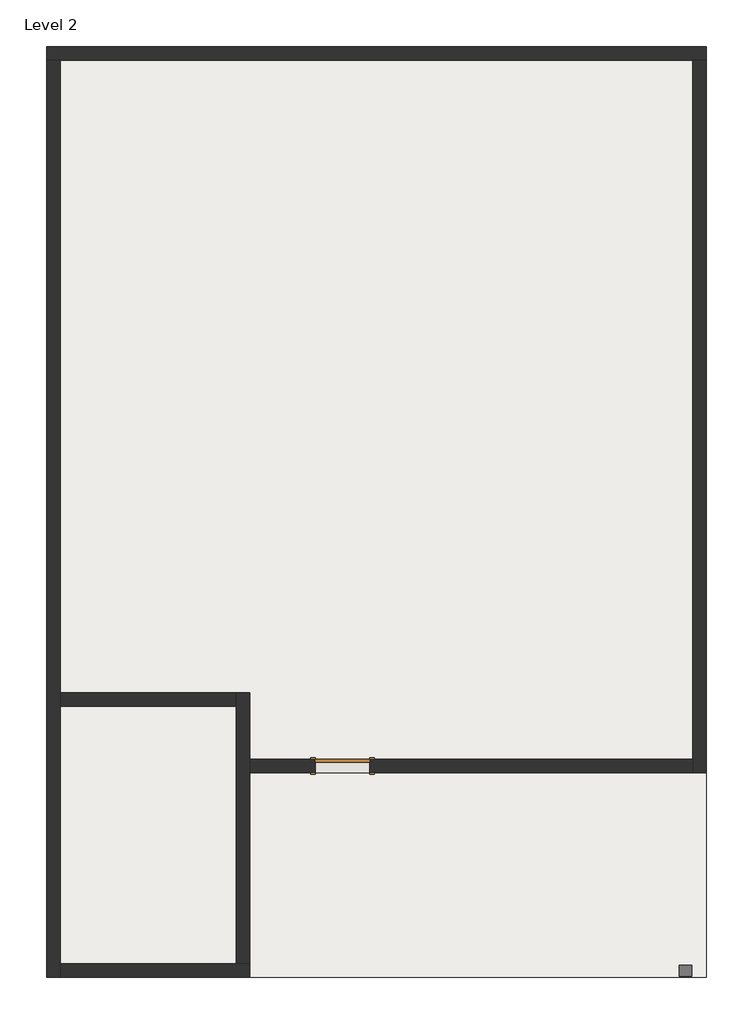
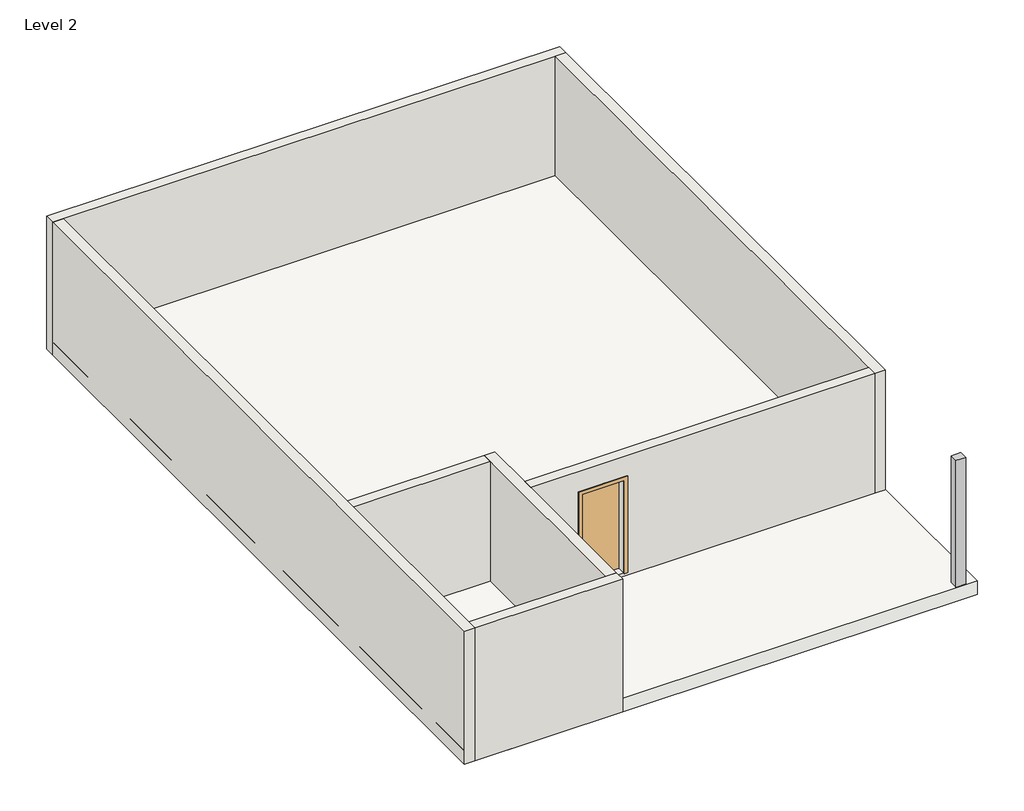
# One storey: 7 walls, 1 door, 1 proxy, 1 roof.
"""IFC4 building model written with IfcOpenShell, lengths in millimetres."""

from ifc_helpers import new_model, si_unit, frame, origin, place, context, project, spatial, polyline, outline, extrude, faceted_brep, transform, mapped, element, save
from components import generic_models_3_generic_models_3_3f4cf848, door_a90ba1ad

model = new_model("IFC4")

# Units and contexts
model_context = context("Model", 3, world=origin())
ifc_project = project(units=[si_unit("LENGTHUNIT", "METRE", prefix="MILLI")], contexts=[model_context])

# Site, building, storey
site = spatial("IfcSite", under=ifc_project)
building = spatial("IfcBuilding", under=site)
storey = spatial("IfcBuildingStorey", under=building, Name="Level 2", Elevation=3048.0)

# Proxy
placement = place(None, origin())
generic_models_3_generic_models_3_shape = generic_models_3_generic_models_3_3f4cf848(model_context)
element("IfcBuildingElementProxy", 1, Name="Generic Models 3 : Generic Models 3", ObjectType="Generic Models 3 : Generic Models 3", at=placement, inside=storey, context=model_context, shape_type="MappedRepresentation", body=[
    mapped(generic_models_3_generic_models_3_shape, transform((0.0, 0.0, 0.0), x_axis=(1.0, 0.0, 0.0), y_axis=(0.0, 1.0, 0.0), z_axis=(0.0, 0.0, 1.0))),
])

# Door
door_shape = door_a90ba1ad(model_context)
element("IfcDoor", 2, ObjectType="Single-Flush : 36\" x 84\"", at=placement, inside=storey, context=model_context, shape_type="MappedRepresentation", body=[
    mapped(door_shape, transform((-12010.0767684, -11765.0742702, 3429.0), x_axis=(-1.0, 0.0, 0.0), y_axis=(0.0, -1.0, 0.0), z_axis=(0.0, 0.0, 1.0))),
])

# Roof
element("IfcRoof", 3, ObjectType="Generic - 12\"", at=placement, inside=storey, context=model_context, shape_type="SweptSolid", body=[
    extrude(outline(polyline([(-17001.1767684, 363.4257298), (-5875.9767684, 363.4257298), (-5875.9767684, -15333.7742702), (-17001.1767684, -15333.7742702), (-17001.1767684, 363.4257298)])), frame((0.0, 0.0, 3048.0), z_axis=(0.0, 0.0, 1.0), x_axis=(1.0, 0.0, 0.0)), (0.0, 0.0, 1.0), 304.8),
])

# Walls
element("IfcWall", 4, ObjectType="9\"", at=placement, inside=storey, context=model_context, shape_type="Brep", body=[
    faceted_brep([(-17001.1767684, 134.8257298, 3048.0), (-16772.5767684, 134.8257298, 3048.0), (-6104.5767684, 134.8257298, 3048.0), (-5875.9767684, 134.8257298, 3048.0), (-5875.9767684, 134.8257298, 6096.0), (-6104.5767684, 134.8257298, 6096.0), (-16772.5767684, 134.8257298, 6096.0), (-17001.1767684, 134.8257298, 6096.0), (-17001.1767684, 363.4257298, 3048.0), (-17001.1767684, 363.4257298, 6096.0), (-5875.9767684, 363.4257298, 6096.0), (-5875.9767684, 363.4257298, 3048.0)], [[[0, 1, 2, 3, 4, 5, 6, 7]], [[8, 9, 10, 11]], [[3, 2, 1, 0, 8, 11]], [[7, 6, 5, 4, 10, 9]], [[4, 3, 11, 10]], [[0, 7, 9, 8]]]),
])
element("IfcWall", 5, ObjectType="9\"", at=placement, inside=storey, context=model_context, shape_type="Brep", body=[
    faceted_brep([(-6104.5767684, 134.8257298, 3048.0), (-6104.5767684, -11650.7742702, 3048.0), (-6104.5767684, -11879.3742702, 3048.0), (-6104.5767684, -11879.3742702, 6096.0), (-6104.5767684, -11650.7742702, 6096.0), (-6104.5767684, 134.8257298, 6096.0), (-5875.9767684, 134.8257298, 3048.0), (-5875.9767684, 134.8257298, 6096.0), (-5875.9767684, -11879.3742702, 6096.0), (-5875.9767684, -11879.3742702, 3048.0)], [[[0, 1, 2, 3, 4, 5]], [[6, 7, 8, 9]], [[2, 1, 0, 6, 9]], [[3, 2, 9, 8]], [[5, 4, 3, 8, 7]], [[0, 5, 7, 6]]]),
])
element("IfcWall", 6, ObjectType="9\"", at=placement, inside=storey, context=model_context, shape_type="Brep", body=[
    faceted_brep([(-16772.5767684, -15333.7742702, 3048.0), (-16772.5767684, -15105.1742702, 3048.0), (-16772.5767684, -10761.7742702, 3048.0), (-16772.5767684, -10533.1742702, 3048.0), (-16772.5767684, 134.8257298, 3048.0), (-16772.5767684, 134.8257298, 6096.0), (-16772.5767684, -10533.1742702, 6096.0), (-16772.5767684, -10761.7742702, 6096.0), (-16772.5767684, -15105.1742702, 6096.0), (-16772.5767684, -15333.7742702, 6096.0), (-17001.1767684, -15333.7742702, 3048.0), (-17001.1767684, -15333.7742702, 6096.0), (-17001.1767684, 134.8257298, 6096.0), (-17001.1767684, 134.8257298, 3048.0)], [[[0, 1, 2, 3, 4, 5, 6, 7, 8, 9]], [[10, 11, 12, 13]], [[4, 3, 2, 1, 0, 10, 13]], [[9, 8, 7, 6, 5, 12, 11]], [[5, 4, 13, 12]], [[0, 9, 11, 10]]]),
])
element("IfcWall", 7, ObjectType="9\"", at=placement, inside=storey, context=model_context, shape_type="Brep", body=[
    faceted_brep([(-16772.5767684, -15333.7742702, 3048.0), (-13572.1767684, -15333.7742702, 3048.0), (-13572.1767684, -15333.7742702, 6096.0), (-16772.5767684, -15333.7742702, 6096.0), (-16772.5767684, -15105.1742702, 3048.0), (-16772.5767684, -15105.1742702, 6096.0), (-13800.7767684, -15105.1742702, 6096.0), (-13572.1767684, -15105.1742702, 6096.0), (-13572.1767684, -15105.1742702, 3048.0), (-13800.7767684, -15105.1742702, 3048.0)], [[[0, 1, 2, 3]], [[4, 5, 6, 7, 8, 9]], [[1, 0, 4, 9, 8]], [[3, 2, 7, 6, 5]], [[0, 3, 5, 4]], [[2, 1, 8, 7]]]),
])
element("IfcWall", 8, ObjectType="9\"", at=placement, inside=storey, context=model_context, shape_type="Brep", body=[
    faceted_brep([(-13572.1767684, -15105.1742702, 3048.0), (-13572.1767684, -11879.3742702, 3048.0), (-13572.1767684, -11650.7742702, 3048.0), (-13572.1767684, -10533.1742702, 3048.0), (-13572.1767684, -10533.1742702, 6096.0), (-13572.1767684, -11650.7742702, 6096.0), (-13572.1767684, -11879.3742702, 6096.0), (-13572.1767684, -15105.1742702, 6096.0), (-13800.7767684, -15105.1742702, 3048.0), (-13800.7767684, -15105.1742702, 6096.0), (-13800.7767684, -10761.7742702, 6096.0), (-13800.7767684, -10533.1742702, 6096.0), (-13800.7767684, -10533.1742702, 3048.0), (-13800.7767684, -10761.7742702, 3048.0)], [[[0, 1, 2, 3, 4, 5, 6, 7]], [[8, 9, 10, 11, 12, 13]], [[3, 2, 1, 0, 8, 13, 12]], [[7, 6, 5, 4, 11, 10, 9]], [[0, 7, 9, 8]], [[4, 3, 12, 11]]]),
])
element("IfcWall", 9, ObjectType="9\"", at=placement, inside=storey, context=model_context, shape_type="SweptSolid", body=[
    extrude(outline(polyline([(-16772.5767684, -10533.1742702), (-13800.7767684, -10533.1742702), (-13800.7767684, -10761.7742702), (-16772.5767684, -10761.7742702), (-16772.5767684, -10533.1742702)])), frame((0.0, 0.0, 3048.0), z_axis=(0.0, 0.0, 1.0), x_axis=(1.0, 0.0, 0.0)), (0.0, 0.0, 1.0), 3048.0),
])
element("IfcWall", 10, ObjectType="9\"", at=placement, inside=storey, context=model_context, shape_type="SweptSolid", body=[
    extrude(outline(polyline([(3048.0, -13572.1767684), (3048.0, -6104.5767684), (6096.0, -6104.5767684), (6096.0, -13572.1767684), (3048.0, -13572.1767684)]), holes=[polyline([(3429.0, -11552.8767684), (3429.0, -12467.2767684), (5562.6, -12467.2767684), (5562.6, -11552.8767684), (3429.0, -11552.8767684)])]), frame((0.0, -11879.3742702, 0.0), z_axis=(0.0, 1.0, 0.0), x_axis=(0.0, 0.0, 1.0)), (0.0, 0.0, 1.0), 228.6),
])

save(model, "model.ifc")

# Revit data of these elements
# Type "Single-Flush : 36\" x 84\""
#   Type Mark = "1"
#   Construction Type Id = "MDOOR"
#   Assembly Code = "C1020"
#   Analytic Construction = "Metal"
#   Thickness = 0' - 2"
#   Heat Transfer Coefficient (U) = 0.651978 BTU/(h·ft²·°F)
#   Height = 7' - 0"
#   Trim Projection Ext = 0' - 1"
#   Trim Projection Int = 0' - 1"
#   Trim Width = 0' - 3"
#   Width = 3' - 0"
#   Define Thermal Properties by = 1
#   Define Thermal Properties by = 1
#   Door Material = Door - Panel
#   Frame Material = Door - Frame
#   Visual Light Transmittance = 0
#   Solar Heat Gain Coefficient = 0
#   Function = (empty or 0)
#   Wall Closure = (empty or 0)
# Type "Generic - 12\""
#   Assembly Code = "B1020"
#   Layers, outside or top first: 1' - 0" no material (function 1)
# Type "9\""
#   Assembly Code = "B2010"
#   Layers, outside or top first: 0' - 9" no material (function 1)
# Element 1 (IfcBuildingElementProxy, "Generic Models 3 : Generic Models 3")
#   Phase Created = New Construction
# Element 2 (IfcDoor, "Single-Flush : 36\" x 84\"")
#   Phase Created = New Construction
#   Materials on its faces: "Door - Frame", "Door - Panel"
# Element 3 (IfcRoof, "Generic - 12\"")
#   built-in parameter 1001705 = 11 (stored number, unit not read)
#   built-in parameter 1001710 = 33615
#   Phase Created = New Construction
#   Materials on its faces: "Default Roof"
# Elements 4, 5, 6, 7, 8, 9, 10 (IfcWall, "9\"")
#   Top Offset = 0' - 0"
#   Base Offset = 0' - 0"
#   Unconnected Height = 10' - 0"
#   wall height = 10' - 0"
#   Phase Created = New Construction
#   Base Constraint = Level 2
#   Materials on its faces: "Default Wall"
# Materials
#   "Door - Panel": class "Wood", colour RGB 210 159 95, transparency 0, Cost = 0
#   "Door - Frame": colour RGB 118 70 51, transparency 0, Cost = 0
#   "Default Roof": colour RGB 88 101 114, transparency 0, Cost = 0
#   "Default Wall": colour RGB 128 128 128, transparency 0, Cost = 0
